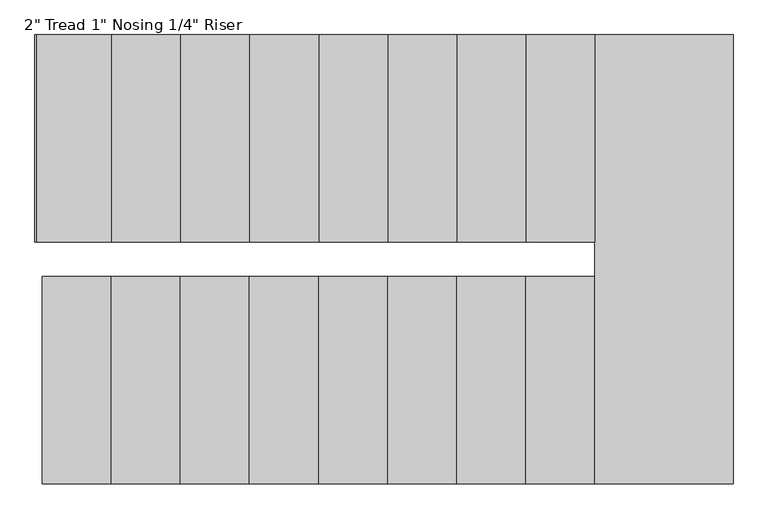
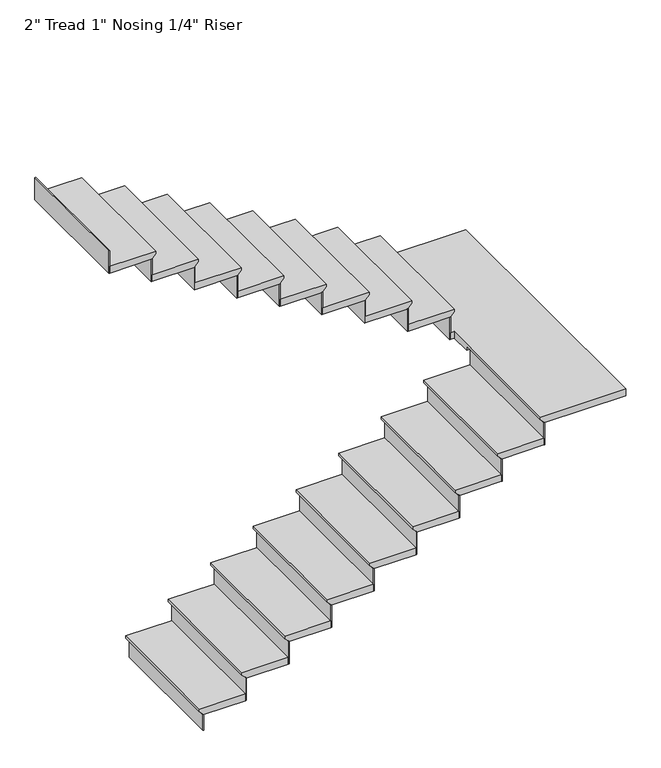
"""IFC4 building model written with IfcOpenShell, lengths in millimetres: stair flight geometry."""

from ifc_helpers import new_model, si_unit, origin, place, context, project, spatial, faceted_brep, source, transform, mapped, element, save


def stair_flight_460b4896(model_context):
    return source(origin(), model_context, "Body", "Brep", [
        faceted_brep([(-1197.97188, -4816.50869, 6398.6833333), (-1197.97188, -4816.50869, 6417.7333333), (-1197.97188, -3902.10869, 6417.7333333), (-1197.97188, -3902.10869, 6398.6833333), (-1172.57188, -4816.50869, 6373.2833333), (-1172.57188, -3902.10869, 6373.2833333), (-867.77188, -4816.50869, 6417.7333333), (-867.77188, -3902.10869, 6417.7333333), (-1172.57188, -3902.10869, 6366.9333333), (-867.77188, -3902.10869, 6366.9333333), (-867.77188, -4816.50869, 6366.9333333), (-1172.57188, -4816.50869, 6366.9333333)], [[[0, 1, 2, 3]], [[4, 0, 3, 5]], [[2, 1, 6, 7]], [[8, 9, 10, 11]], [[2, 7, 9, 8, 5, 3]], [[8, 11, 4, 5]], [[6, 1, 0, 4, 11, 10]], [[7, 6, 10, 9]]]),
        faceted_brep([(-1172.57188, -4816.50869, 6366.9333333), (-1172.57188, -4816.50869, 6248.4), (-1166.22188, -4816.50869, 6248.4), (-1166.22188, -4816.50869, 6366.9333333), (-1172.57188, -3902.10869, 6366.9333333), (-1166.22188, -3902.10869, 6366.9333333), (-1166.22188, -3902.10869, 6248.4), (-1172.57188, -3902.10869, 6248.4)], [[[0, 1, 2, 3]], [[4, 5, 6, 7]], [[1, 0, 4, 7]], [[2, 1, 7, 6]], [[3, 2, 6, 5]], [[0, 3, 5, 4]]]),
        faceted_brep([(-867.77188, -4816.50869, 6536.2666667), (-867.77188, -4816.50869, 6366.9333333), (-861.42188, -4816.50869, 6366.9333333), (-861.42188, -4816.50869, 6536.2666667), (-867.77188, -3902.10869, 6536.2666667), (-861.42188, -3902.10869, 6536.2666667), (-861.42188, -3902.10869, 6366.9333333), (-867.77188, -3902.10869, 6366.9333333)], [[[0, 1, 2, 3]], [[4, 5, 6, 7]], [[1, 0, 4, 7]], [[2, 1, 7, 6]], [[3, 2, 6, 5]], [[0, 3, 5, 4]]]),
        faceted_brep([(-893.17188, -3902.10869, 6587.0666667), (-893.17188, -4816.50869, 6587.0666667), (-562.97188, -4816.50869, 6587.0666667), (-562.97188, -3902.10869, 6587.0666667), (-867.77188, -3902.10869, 6536.2666667), (-562.97188, -3902.10869, 6536.2666667), (-562.97188, -4816.50869, 6536.2666667), (-867.77188, -4816.50869, 6536.2666667), (-867.77188, -3902.10869, 6542.6166667), (-893.17188, -3902.10869, 6568.0166667), (-867.77188, -4816.50869, 6542.6166667), (-893.17188, -4816.50869, 6568.0166667)], [[[0, 1, 2, 3]], [[4, 5, 6, 7]], [[0, 3, 5, 4, 8, 9]], [[4, 7, 10, 8]], [[2, 1, 11, 10, 7, 6]], [[3, 2, 6, 5]], [[11, 1, 0, 9]], [[10, 11, 9, 8]]]),
        faceted_brep([(-562.97188, -4816.50869, 6705.6), (-562.97188, -4816.50869, 6536.2666667), (-556.62188, -4816.50869, 6536.2666667), (-556.62188, -4816.50869, 6705.6), (-562.97188, -3902.10869, 6705.6), (-556.62188, -3902.10869, 6705.6), (-556.62188, -3902.10869, 6536.2666667), (-562.97188, -3902.10869, 6536.2666667)], [[[0, 1, 2, 3]], [[4, 5, 6, 7]], [[1, 0, 4, 7]], [[2, 1, 7, 6]], [[3, 2, 6, 5]], [[0, 3, 5, 4]]]),
        faceted_brep([(-588.37188, -3902.10869, 6756.4), (-588.37188, -4816.50869, 6756.4), (-258.17188, -4816.50869, 6756.4), (-258.17188, -3902.10869, 6756.4), (-562.97188, -3902.10869, 6705.6), (-258.17188, -3902.10869, 6705.6), (-258.17188, -4816.50869, 6705.6), (-562.97188, -4816.50869, 6705.6), (-562.97188, -3902.10869, 6711.95), (-588.37188, -3902.10869, 6737.35), (-562.97188, -4816.50869, 6711.95), (-588.37188, -4816.50869, 6737.35)], [[[0, 1, 2, 3]], [[4, 5, 6, 7]], [[0, 3, 5, 4, 8, 9]], [[4, 7, 10, 8]], [[2, 1, 11, 10, 7, 6]], [[3, 2, 6, 5]], [[11, 1, 0, 9]], [[10, 11, 9, 8]]]),
        faceted_brep([(-258.17188, -4816.50869, 6874.9333333), (-258.17188, -4816.50869, 6705.6), (-251.82188, -4816.50869, 6705.6), (-251.82188, -4816.50869, 6874.9333333), (-258.17188, -3902.10869, 6874.9333333), (-251.82188, -3902.10869, 6874.9333333), (-251.82188, -3902.10869, 6705.6), (-258.17188, -3902.10869, 6705.6)], [[[0, 1, 2, 3]], [[4, 5, 6, 7]], [[1, 0, 4, 7]], [[2, 1, 7, 6]], [[3, 2, 6, 5]], [[0, 3, 5, 4]]]),
        faceted_brep([(-283.57188, -3902.10869, 6925.7333333), (-283.57188, -4816.50869, 6925.7333333), (46.62812, -4816.50869, 6925.7333333), (46.62812, -3902.10869, 6925.7333333), (-258.17188, -3902.10869, 6874.9333333), (46.62812, -3902.10869, 6874.9333333), (46.62812, -4816.50869, 6874.9333333), (-258.17188, -4816.50869, 6874.9333333), (-258.17188, -3902.10869, 6881.2833333), (-283.57188, -3902.10869, 6906.6833333), (-258.17188, -4816.50869, 6881.2833333), (-283.57188, -4816.50869, 6906.6833333)], [[[0, 1, 2, 3]], [[4, 5, 6, 7]], [[0, 3, 5, 4, 8, 9]], [[4, 7, 10, 8]], [[2, 1, 11, 10, 7, 6]], [[3, 2, 6, 5]], [[11, 1, 0, 9]], [[10, 11, 9, 8]]]),
        faceted_brep([(46.62812, -4816.50869, 7044.2666667), (46.62812, -4816.50869, 6874.9333333), (52.97812, -4816.50869, 6874.9333333), (52.97812, -4816.50869, 7044.2666667), (46.62812, -3902.10869, 7044.2666667), (52.97812, -3902.10869, 7044.2666667), (52.97812, -3902.10869, 6874.9333333), (46.62812, -3902.10869, 6874.9333333)], [[[0, 1, 2, 3]], [[4, 5, 6, 7]], [[1, 0, 4, 7]], [[2, 1, 7, 6]], [[3, 2, 6, 5]], [[0, 3, 5, 4]]]),
        faceted_brep([(21.22812, -3902.10869, 7095.0666667), (21.22812, -4816.50869, 7095.0666667), (351.42812, -4816.50869, 7095.0666667), (351.42812, -3902.10869, 7095.0666667), (46.62812, -3902.10869, 7044.2666667), (351.42812, -3902.10869, 7044.2666667), (351.42812, -4816.50869, 7044.2666667), (46.62812, -4816.50869, 7044.2666667), (46.62812, -3902.10869, 7050.6166667), (21.22812, -3902.10869, 7076.0166667), (46.62812, -4816.50869, 7050.6166667), (21.22812, -4816.50869, 7076.0166667)], [[[0, 1, 2, 3]], [[4, 5, 6, 7]], [[0, 3, 5, 4, 8, 9]], [[4, 7, 10, 8]], [[2, 1, 11, 10, 7, 6]], [[3, 2, 6, 5]], [[11, 1, 0, 9]], [[10, 11, 9, 8]]]),
        faceted_brep([(351.42812, -4816.50869, 7213.6), (351.42812, -4816.50869, 7044.2666667), (357.77812, -4816.50869, 7044.2666667), (357.77812, -4816.50869, 7213.6), (351.42812, -3902.10869, 7213.6), (357.77812, -3902.10869, 7213.6), (357.77812, -3902.10869, 7044.2666667), (351.42812, -3902.10869, 7044.2666667)], [[[0, 1, 2, 3]], [[4, 5, 6, 7]], [[1, 0, 4, 7]], [[2, 1, 7, 6]], [[3, 2, 6, 5]], [[0, 3, 5, 4]]]),
        faceted_brep([(326.02812, -3902.10869, 7264.4), (326.02812, -4816.50869, 7264.4), (656.22812, -4816.50869, 7264.4), (656.22812, -3902.10869, 7264.4), (351.42812, -3902.10869, 7213.6), (656.22812, -3902.10869, 7213.6), (656.22812, -4816.50869, 7213.6), (351.42812, -4816.50869, 7213.6), (351.42812, -3902.10869, 7219.95), (326.02812, -3902.10869, 7245.35), (351.42812, -4816.50869, 7219.95), (326.02812, -4816.50869, 7245.35)], [[[0, 1, 2, 3]], [[4, 5, 6, 7]], [[0, 3, 5, 4, 8, 9]], [[4, 7, 10, 8]], [[2, 1, 11, 10, 7, 6]], [[3, 2, 6, 5]], [[11, 1, 0, 9]], [[10, 11, 9, 8]]]),
        faceted_brep([(656.22812, -4816.50869, 7382.9333333), (656.22812, -4816.50869, 7213.6), (662.57812, -4816.50869, 7213.6), (662.57812, -4816.50869, 7382.9333333), (656.22812, -3902.10869, 7382.9333333), (662.57812, -3902.10869, 7382.9333333), (662.57812, -3902.10869, 7213.6), (656.22812, -3902.10869, 7213.6)], [[[0, 1, 2, 3]], [[4, 5, 6, 7]], [[1, 0, 4, 7]], [[2, 1, 7, 6]], [[3, 2, 6, 5]], [[0, 3, 5, 4]]]),
        faceted_brep([(630.82812, -3902.10869, 7433.7333333), (630.82812, -4816.50869, 7433.7333333), (961.02812, -4816.50869, 7433.7333333), (961.02812, -3902.10869, 7433.7333333), (656.22812, -3902.10869, 7382.9333333), (961.02812, -3902.10869, 7382.9333333), (961.02812, -4816.50869, 7382.9333333), (656.22812, -4816.50869, 7382.9333333), (656.22812, -3902.10869, 7389.2833333), (630.82812, -3902.10869, 7414.6833333), (656.22812, -4816.50869, 7389.2833333), (630.82812, -4816.50869, 7414.6833333)], [[[0, 1, 2, 3]], [[4, 5, 6, 7]], [[0, 3, 5, 4, 8, 9]], [[4, 7, 10, 8]], [[2, 1, 11, 10, 7, 6]], [[3, 2, 6, 5]], [[11, 1, 0, 9]], [[10, 11, 9, 8]]]),
        faceted_brep([(961.02812, -4816.50869, 7552.2666667), (961.02812, -4816.50869, 7382.9333333), (967.37812, -4816.50869, 7382.9333333), (967.37812, -4816.50869, 7552.2666667), (961.02812, -3902.10869, 7552.2666667), (967.37812, -3902.10869, 7552.2666667), (967.37812, -3902.10869, 7382.9333333), (961.02812, -3902.10869, 7382.9333333)], [[[0, 1, 2, 3]], [[4, 5, 6, 7]], [[1, 0, 4, 7]], [[2, 1, 7, 6]], [[3, 2, 6, 5]], [[0, 3, 5, 4]]]),
        faceted_brep([(935.62812, -3902.10869, 7603.0666667), (935.62812, -4816.50869, 7603.0666667), (1265.82812, -4816.50869, 7603.0666667), (1265.82812, -3902.10869, 7603.0666667), (961.02812, -3902.10869, 7552.2666667), (1265.82812, -3902.10869, 7552.2666667), (1265.82812, -4816.50869, 7552.2666667), (961.02812, -4816.50869, 7552.2666667), (961.02812, -3902.10869, 7558.6166667), (935.62812, -3902.10869, 7584.0166667), (961.02812, -4816.50869, 7558.6166667), (935.62812, -4816.50869, 7584.0166667)], [[[0, 1, 2, 3]], [[4, 5, 6, 7]], [[0, 3, 5, 4, 8, 9]], [[4, 7, 10, 8]], [[2, 1, 11, 10, 7, 6]], [[3, 2, 6, 5]], [[11, 1, 0, 9]], [[10, 11, 9, 8]]]),
        faceted_brep([(1265.82812, -4816.50869, 7721.6), (1265.82812, -4816.50869, 7552.2666667), (1272.17812, -4816.50869, 7552.2666667), (1272.17812, -4816.50869, 7721.6), (1265.82812, -3902.10869, 7721.6), (1272.17812, -3902.10869, 7721.6), (1272.17812, -3902.10869, 7552.2666667), (1265.82812, -3902.10869, 7552.2666667)], [[[0, 1, 2, 3]], [[4, 5, 6, 7]], [[1, 0, 4, 7]], [[2, 1, 7, 6]], [[3, 2, 6, 5]], [[0, 3, 5, 4]]]),
        faceted_brep([(1215.02812, -3749.70869, 7772.4), (1240.42812, -3749.70869, 7772.4), (1240.42812, -4816.50869, 7772.4), (1850.02812, -4816.50869, 7772.4), (1850.02812, -2835.30869, 7772.4), (1215.02812, -2835.30869, 7772.4), (1240.42812, -3749.70869, 7721.6), (1215.02812, -3749.70869, 7721.6), (1215.02812, -2835.30869, 7721.6), (1850.02812, -2835.30869, 7721.6), (1850.02812, -4816.50869, 7721.6), (1265.82812, -4816.50869, 7721.6), (1265.82812, -3902.10869, 7721.6), (1240.42812, -3902.10869, 7721.6), (1240.42812, -3902.10869, 7753.35), (1240.42812, -4816.50869, 7753.35), (1265.82812, -3902.10869, 7727.95), (1265.82812, -4816.50869, 7727.95)], [[[0, 1, 2, 3, 4, 5]], [[6, 7, 8, 9, 10, 11, 12, 13]], [[1, 0, 7, 6]], [[2, 1, 6, 13, 14, 15]], [[13, 12, 16, 14]], [[12, 11, 17, 16]], [[3, 2, 15, 17, 11, 10]], [[4, 3, 10, 9]], [[5, 4, 9, 8]], [[0, 5, 8, 7]], [[17, 15, 14, 16]]]),
        faceted_brep([(1215.02812, -2835.30869, 7890.9333333), (1215.02812, -2835.30869, 7721.6), (1208.67812, -2835.30869, 7721.6), (1208.67812, -2835.30869, 7890.9333333), (1215.02812, -3749.70869, 7890.9333333), (1208.67812, -3749.70869, 7890.9333333), (1208.67812, -3749.70869, 7721.6), (1215.02812, -3749.70869, 7721.6)], [[[0, 1, 2, 3]], [[4, 5, 6, 7]], [[1, 0, 4, 7]], [[2, 1, 7, 6]], [[3, 2, 6, 5]], [[0, 3, 5, 4]]]),
        faceted_brep([(1240.42812, -3749.70869, 7941.7333333), (1240.42812, -2835.30869, 7941.7333333), (910.22812, -2835.30869, 7941.7333333), (910.22812, -3749.70869, 7941.7333333), (1215.02812, -3749.70869, 7890.9333333), (910.22812, -3749.70869, 7890.9333333), (910.22812, -2835.30869, 7890.9333333), (1215.02812, -2835.30869, 7890.9333333), (1215.02812, -3749.70869, 7897.2833333), (1240.42812, -3749.70869, 7922.6833333), (1215.02812, -2835.30869, 7897.2833333), (1240.42812, -2835.30869, 7922.6833333)], [[[0, 1, 2, 3]], [[4, 5, 6, 7]], [[0, 3, 5, 4, 8, 9]], [[4, 7, 10, 8]], [[2, 1, 11, 10, 7, 6]], [[3, 2, 6, 5]], [[11, 1, 0, 9]], [[10, 11, 9, 8]]]),
        faceted_brep([(910.22812, -2835.30869, 8060.2666667), (910.22812, -2835.30869, 7890.9333333), (903.87812, -2835.30869, 7890.9333333), (903.87812, -2835.30869, 8060.2666667), (910.22812, -3749.70869, 8060.2666667), (903.87812, -3749.70869, 8060.2666667), (903.87812, -3749.70869, 7890.9333333), (910.22812, -3749.70869, 7890.9333333)], [[[0, 1, 2, 3]], [[4, 5, 6, 7]], [[1, 0, 4, 7]], [[2, 1, 7, 6]], [[3, 2, 6, 5]], [[0, 3, 5, 4]]]),
        faceted_brep([(935.62812, -3749.70869, 8111.0666667), (935.62812, -2835.30869, 8111.0666667), (605.42812, -2835.30869, 8111.0666667), (605.42812, -3749.70869, 8111.0666667), (910.22812, -3749.70869, 8060.2666667), (605.42812, -3749.70869, 8060.2666667), (605.42812, -2835.30869, 8060.2666667), (910.22812, -2835.30869, 8060.2666667), (910.22812, -3749.70869, 8066.6166667), (935.62812, -3749.70869, 8092.0166667), (910.22812, -2835.30869, 8066.6166667), (935.62812, -2835.30869, 8092.0166667)], [[[0, 1, 2, 3]], [[4, 5, 6, 7]], [[0, 3, 5, 4, 8, 9]], [[4, 7, 10, 8]], [[2, 1, 11, 10, 7, 6]], [[3, 2, 6, 5]], [[11, 1, 0, 9]], [[10, 11, 9, 8]]]),
        faceted_brep([(605.42812, -2835.30869, 8229.6), (605.42812, -2835.30869, 8060.2666667), (599.07812, -2835.30869, 8060.2666667), (599.07812, -2835.30869, 8229.6), (605.42812, -3749.70869, 8229.6), (599.07812, -3749.70869, 8229.6), (599.07812, -3749.70869, 8060.2666667), (605.42812, -3749.70869, 8060.2666667)], [[[0, 1, 2, 3]], [[4, 5, 6, 7]], [[1, 0, 4, 7]], [[2, 1, 7, 6]], [[3, 2, 6, 5]], [[0, 3, 5, 4]]]),
        faceted_brep([(630.82812, -3749.70869, 8280.4), (630.82812, -2835.30869, 8280.4), (300.62812, -2835.30869, 8280.4), (300.62812, -3749.70869, 8280.4), (605.42812, -3749.70869, 8229.6), (300.62812, -3749.70869, 8229.6), (300.62812, -2835.30869, 8229.6), (605.42812, -2835.30869, 8229.6), (605.42812, -3749.70869, 8235.95), (630.82812, -3749.70869, 8261.35), (605.42812, -2835.30869, 8235.95), (630.82812, -2835.30869, 8261.35)], [[[0, 1, 2, 3]], [[4, 5, 6, 7]], [[0, 3, 5, 4, 8, 9]], [[4, 7, 10, 8]], [[2, 1, 11, 10, 7, 6]], [[3, 2, 6, 5]], [[11, 1, 0, 9]], [[10, 11, 9, 8]]]),
        faceted_brep([(300.62812, -2835.30869, 8398.9333333), (300.62812, -2835.30869, 8229.6), (294.27812, -2835.30869, 8229.6), (294.27812, -2835.30869, 8398.9333333), (300.62812, -3749.70869, 8398.9333333), (294.27812, -3749.70869, 8398.9333333), (294.27812, -3749.70869, 8229.6), (300.62812, -3749.70869, 8229.6)], [[[0, 1, 2, 3]], [[4, 5, 6, 7]], [[1, 0, 4, 7]], [[2, 1, 7, 6]], [[3, 2, 6, 5]], [[0, 3, 5, 4]]]),
        faceted_brep([(326.02812, -3749.70869, 8449.7333333), (326.02812, -2835.30869, 8449.7333333), (-4.17188, -2835.30869, 8449.7333333), (-4.17188, -3749.70869, 8449.7333333), (300.62812, -3749.70869, 8398.9333333), (-4.17188, -3749.70869, 8398.9333333), (-4.17188, -2835.30869, 8398.9333333), (300.62812, -2835.30869, 8398.9333333), (300.62812, -3749.70869, 8405.2833333), (326.02812, -3749.70869, 8430.6833333), (300.62812, -2835.30869, 8405.2833333), (326.02812, -2835.30869, 8430.6833333)], [[[0, 1, 2, 3]], [[4, 5, 6, 7]], [[0, 3, 5, 4, 8, 9]], [[4, 7, 10, 8]], [[2, 1, 11, 10, 7, 6]], [[3, 2, 6, 5]], [[11, 1, 0, 9]], [[10, 11, 9, 8]]]),
        faceted_brep([(-4.17188, -2835.30869, 8568.2666667), (-4.17188, -2835.30869, 8398.9333333), (-10.52188, -2835.30869, 8398.9333333), (-10.52188, -2835.30869, 8568.2666667), (-4.17188, -3749.70869, 8568.2666667), (-10.52188, -3749.70869, 8568.2666667), (-10.52188, -3749.70869, 8398.9333333), (-4.17188, -3749.70869, 8398.9333333)], [[[0, 1, 2, 3]], [[4, 5, 6, 7]], [[1, 0, 4, 7]], [[2, 1, 7, 6]], [[3, 2, 6, 5]], [[0, 3, 5, 4]]]),
        faceted_brep([(21.22812, -3749.70869, 8619.0666667), (21.22812, -2835.30869, 8619.0666667), (-308.97188, -2835.30869, 8619.0666667), (-308.97188, -3749.70869, 8619.0666667), (-4.17188, -3749.70869, 8568.2666667), (-308.97188, -3749.70869, 8568.2666667), (-308.97188, -2835.30869, 8568.2666667), (-4.17188, -2835.30869, 8568.2666667), (-4.17188, -3749.70869, 8574.6166667), (21.22812, -3749.70869, 8600.0166667), (-4.17188, -2835.30869, 8574.6166667), (21.22812, -2835.30869, 8600.0166667)], [[[0, 1, 2, 3]], [[4, 5, 6, 7]], [[0, 3, 5, 4, 8, 9]], [[4, 7, 10, 8]], [[2, 1, 11, 10, 7, 6]], [[3, 2, 6, 5]], [[11, 1, 0, 9]], [[10, 11, 9, 8]]]),
        faceted_brep([(-308.97188, -2835.30869, 8737.6), (-308.97188, -2835.30869, 8568.2666667), (-315.32188, -2835.30869, 8568.2666667), (-315.32188, -2835.30869, 8737.6), (-308.97188, -3749.70869, 8737.6), (-315.32188, -3749.70869, 8737.6), (-315.32188, -3749.70869, 8568.2666667), (-308.97188, -3749.70869, 8568.2666667)], [[[0, 1, 2, 3]], [[4, 5, 6, 7]], [[1, 0, 4, 7]], [[2, 1, 7, 6]], [[3, 2, 6, 5]], [[0, 3, 5, 4]]]),
        faceted_brep([(-283.57188, -3749.70869, 8788.4), (-283.57188, -2835.30869, 8788.4), (-613.77188, -2835.30869, 8788.4), (-613.77188, -3749.70869, 8788.4), (-308.97188, -3749.70869, 8737.6), (-613.77188, -3749.70869, 8737.6), (-613.77188, -2835.30869, 8737.6), (-308.97188, -2835.30869, 8737.6), (-308.97188, -3749.70869, 8743.95), (-283.57188, -3749.70869, 8769.35), (-308.97188, -2835.30869, 8743.95), (-283.57188, -2835.30869, 8769.35)], [[[0, 1, 2, 3]], [[4, 5, 6, 7]], [[0, 3, 5, 4, 8, 9]], [[4, 7, 10, 8]], [[2, 1, 11, 10, 7, 6]], [[3, 2, 6, 5]], [[11, 1, 0, 9]], [[10, 11, 9, 8]]]),
        faceted_brep([(-613.77188, -2835.30869, 8906.9333333), (-613.77188, -2835.30869, 8737.6), (-620.12188, -2835.30869, 8737.6), (-620.12188, -2835.30869, 8906.9333333), (-613.77188, -3749.70869, 8906.9333333), (-620.12188, -3749.70869, 8906.9333333), (-620.12188, -3749.70869, 8737.6), (-613.77188, -3749.70869, 8737.6)], [[[0, 1, 2, 3]], [[4, 5, 6, 7]], [[1, 0, 4, 7]], [[2, 1, 7, 6]], [[3, 2, 6, 5]], [[0, 3, 5, 4]]]),
        faceted_brep([(-588.37188, -3749.70869, 8957.7333333), (-588.37188, -2835.30869, 8957.7333333), (-918.57188, -2835.30869, 8957.7333333), (-918.57188, -3749.70869, 8957.7333333), (-613.77188, -3749.70869, 8906.9333333), (-918.57188, -3749.70869, 8906.9333333), (-918.57188, -2835.30869, 8906.9333333), (-613.77188, -2835.30869, 8906.9333333), (-613.77188, -3749.70869, 8913.2833333), (-588.37188, -3749.70869, 8938.6833333), (-613.77188, -2835.30869, 8913.2833333), (-588.37188, -2835.30869, 8938.6833333)], [[[0, 1, 2, 3]], [[4, 5, 6, 7]], [[0, 3, 5, 4, 8, 9]], [[4, 7, 10, 8]], [[2, 1, 11, 10, 7, 6]], [[3, 2, 6, 5]], [[11, 1, 0, 9]], [[10, 11, 9, 8]]]),
        faceted_brep([(-918.57188, -2835.30869, 9076.2666667), (-918.57188, -2835.30869, 8906.9333333), (-924.92188, -2835.30869, 8906.9333333), (-924.92188, -2835.30869, 9076.2666667), (-918.57188, -3749.70869, 9076.2666667), (-924.92188, -3749.70869, 9076.2666667), (-924.92188, -3749.70869, 8906.9333333), (-918.57188, -3749.70869, 8906.9333333)], [[[0, 1, 2, 3]], [[4, 5, 6, 7]], [[1, 0, 4, 7]], [[2, 1, 7, 6]], [[3, 2, 6, 5]], [[0, 3, 5, 4]]]),
        faceted_brep([(-1223.37188, -2835.30869, 9245.6), (-1223.37188, -2835.30869, 9076.2666667), (-1229.72188, -2835.30869, 9076.2666667), (-1229.72188, -2835.30869, 9245.6), (-1223.37188, -3749.70869, 9245.6), (-1229.72188, -3749.70869, 9245.6), (-1229.72188, -3749.70869, 9076.2666667), (-1223.37188, -3749.70869, 9076.2666667)], [[[0, 1, 2, 3]], [[4, 5, 6, 7]], [[1, 0, 4, 7]], [[2, 1, 7, 6]], [[3, 2, 6, 5]], [[0, 3, 5, 4]]]),
        faceted_brep([(-893.17188, -3749.70869, 9127.0666667), (-893.17188, -2835.30869, 9127.0666667), (-1223.37188, -2835.30869, 9127.0666667), (-1223.37188, -3749.70869, 9127.0666667), (-918.57188, -3749.70869, 9076.2666667), (-1223.37188, -3749.70869, 9076.2666667), (-1223.37188, -2835.30869, 9076.2666667), (-918.57188, -2835.30869, 9076.2666667), (-918.57188, -3749.70869, 9082.6166667), (-893.17188, -3749.70869, 9108.0166667), (-918.57188, -2835.30869, 9082.6166667), (-893.17188, -2835.30869, 9108.0166667)], [[[0, 1, 2, 3]], [[4, 5, 6, 7]], [[0, 3, 5, 4, 8, 9]], [[4, 7, 10, 8]], [[2, 1, 11, 10, 7, 6]], [[3, 2, 6, 5]], [[11, 1, 0, 9]], [[10, 11, 9, 8]]]),
    ])


if __name__ == "__main__":
    model = new_model("IFC4")
    model_context = context("Model", 3, world=origin())
    ifc_project = project(units=[si_unit("LENGTHUNIT", "METRE", prefix="MILLI")], contexts=[model_context])
    site = spatial("IfcSite", under=ifc_project)
    building = spatial("IfcBuilding", under=site)
    placement = place(None, origin())
    stair_flight_shape = stair_flight_460b4896(model_context)
    element("IfcStairFlight", 1, ObjectType="2\" Tread 1\" Nosing 1/4\" Riser", at=placement, inside=building, context=model_context, shape_type="MappedRepresentation", body=[
        mapped(stair_flight_shape, transform((0.0, 0.0, 0.0), x_axis=(1.0, 0.0, 0.0), y_axis=(0.0, 1.0, 0.0), z_axis=(0.0, 0.0, 1.0))),
    ])
    save(model, "model.ifc")
